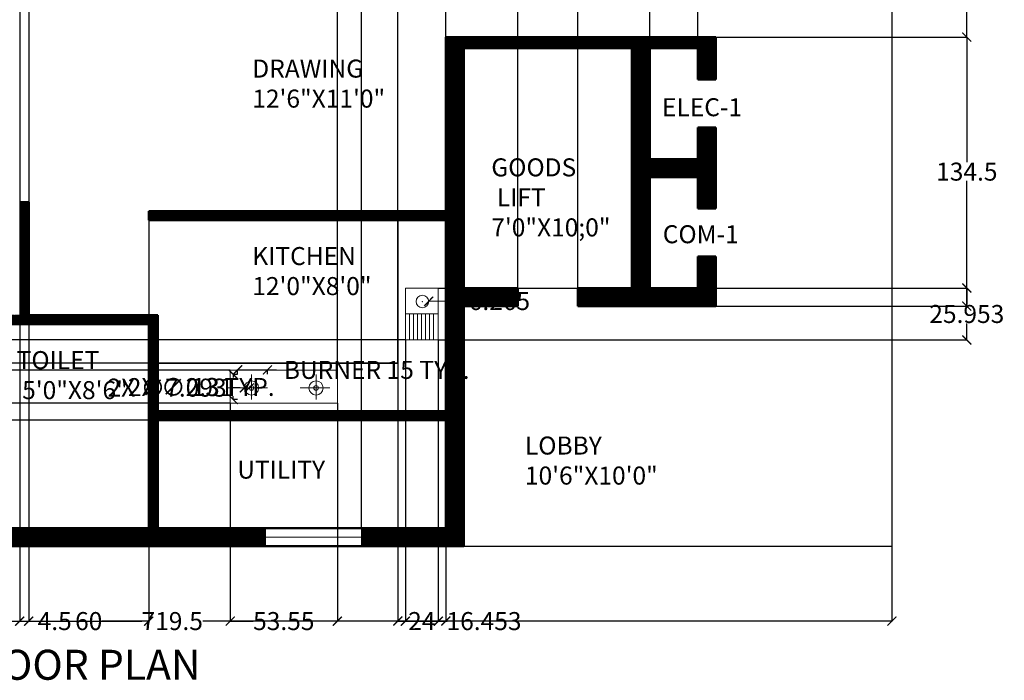
# Model space of a CAD drawing. Units: inches. Extents: x 273 to 1105, y 406 to 1027.
# Tile 2 of 3: x 612 to 1105, y 406 to 736. Entities that reach past the tile are written whole.
import ezdxf

# ---------------------------------------------------------------- set-up
doc = ezdxf.new("R2010")
doc.units = ezdxf.units.IN
doc.header["$MEASUREMENT"] = 0
for name, color, linetype, lineweight in [('A-ANNO-DIMS', 2, 'Continuous', 18), ('A-ANNO-TEXT', 7, 'Continuous', 25), ('A-AREA-IDEN', 7, 'Continuous', 18), ('A-EQPM', 8, 'Continuous', 18), ('A-FIXT-PATT', 8, 'Continuous', 13), ('A-FLOR-CASE', 8, 'Continuous', 25), ('A-FLOR-FIXT', 8, 'Continuous', 18), ('A-FLOR-OTLN', 7, 'Continuous', 25), ('A-GLAZ', 4, 'Continuous', 18), ('A-WALL', 7, 'Continuous', 50), ('A-WALL-PATT', 252, 'Continuous', 13)]:
    doc.layers.add(name, color=color, linetype=linetype, lineweight=lineweight)
doc.styles.get("Standard").update_dxf_attribs({"font": 'arial.ttf'})
doc.dimstyles.get("Standard").update_dxf_attribs({"dimtxt": 9, "dimasz": 4.5, "dimexe": 0.18, "dimexo": 0.0625, "dimgap": 0.09, "dimtad": 0, "dimtih": 1, "dimtoh": 1, "dimdec": 1, "dimzin": 0, "dimdsep": 46, "dimlunit": 4, "dimtxsty": 'Standard', "dimblk": 'ARCHTICK', "dimcen": 0.09, "dimadec": 0, "dimazin": 0, "dimtfac": 1, "dimtdec": 1, "dimtofl": 0, "dimtmove": 0, "dimatfit": 3, "dimfxl": 1, "dimtolj": 1, "dimtzin": 0, "dimarcsym": 0})

# ---------------------------------------------------------------- blocks, each defined once
blk = doc.blocks.new('WIN-48')
for p, q in [((0, 9), (48, 9)), ((0, 0), (0, 9)), ((48, 9), (48, 0)), ((0, 4.5), (48, 4.5)), ((48, 0), (0, 0))]:
    blk.add_line(p, q)
blk = doc.blocks.new('COOKTOP-BURNER')
for p, q in [((6.91, 5.79), (6.91, 12.57)), ((14.89, 5.79), (0, 5.79)), ((0, 5.79), (6.91, 5.79)), ((6.91, 5.79), (6.91, 5.79)), ((6.91, 5.79), (14.89, 5.79)), ((6.91, 5.79), (6.91, 5.79)), ((6.91, 5.79), (6.91, 5.79)), ((6.91, 5.79), (6.91, 5.79)), ((6.91, 5.79), (6.91, 0)), ((6.91, 0), (6.91, 5.79))]:
    blk.add_line(p, q)
for radius in [3.55, 1.16]:
    blk.add_circle((6.91, 5.79), radius)
blk = doc.blocks.new('_ArchTick')
at = {"color": 0, "linetype": 'ByBlock', "const_width": 0.15}
blk.add_lwpolyline([(-0.5, -0.5), (0.5, 0.5)], dxfattribs=at)
blk = doc.blocks.new('*D12')
at = {"layer": 'A-ANNO-DIMS', "color": 0, "lineweight": -2, "transparency": 16777216}
for p, q in [((721.33, 558.55), (721.33, 560.9)), ((721.33, 560.72), (736.23, 560.72)), ((736.23, 558.55), (736.23, 560.9)), ((736.23, 560.72), (740.73, 560.72))]:
    blk.add_line(p, q, dxfattribs=at)
at = {"layer": 'Defpoints', "color": 0, "transparency": 16777216}
for p in [(721.33, 558.49), (736.23, 560.72), (736.23, 558.49)]:
    blk.add_point(p, dxfattribs=at)
at = {"layer": 'A-ANNO-DIMS', "color": 0, "lineweight": -2, "transparency": 16777216, "xscale": 4.5, "yscale": 4.5, "zscale": 4.5, "rotation": 180}
blk.add_blockref('_ArchTick', (721.33, 560.72), dxfattribs=at)
at = {"layer": 'A-ANNO-DIMS', "color": 0, "lineweight": -2, "transparency": 16777216, "xscale": 4.5, "yscale": 4.5, "zscale": 4.5}
blk.add_blockref('_ArchTick', (736.23, 560.72), dxfattribs=at)
at = {"layer": 'A-ANNO-DIMS', "color": 0, "transparency": 16777216, "insert": (790.82, 560.72), "char_height": 9, "attachment_point": 5}
blk.add_mtext('\\A1;BURNER 15 TYP.', dxfattribs=at)
blk = doc.blocks.new('*D13')
at = {"layer": 'A-ANNO-DIMS', "color": 0, "lineweight": -2, "transparency": 16777216}
for p, q in [((721.27, 558.49), (718.92, 558.49)), ((719.1, 558.49), (719.1, 556.89)), ((719.1, 545.92), (719.1, 547.51)), ((721.27, 545.92), (718.92, 545.92))]:
    blk.add_line(p, q, dxfattribs=at)
at = {"layer": 'Defpoints', "color": 0, "transparency": 16777216}
for p in [(719.1, 558.49), (721.33, 558.49), (721.33, 545.92)]:
    blk.add_point(p, dxfattribs=at)
at = {"layer": 'A-ANNO-DIMS', "color": 0, "lineweight": -2, "transparency": 16777216, "xscale": 4.5, "yscale": 4.5, "zscale": 4.5}
for p, rotation in [((719.1, 558.49), 90), ((719.1, 545.92), 270)]:
    blk.add_blockref('_ArchTick', p, dxfattribs=dict(at, rotation=rotation))
at = {"layer": 'A-ANNO-DIMS', "color": 0, "transparency": 16777216, "insert": (719.1, 552.2), "char_height": 9, "attachment_point": 5}
blk.add_mtext('\\A1;13 TYP.', dxfattribs=at)
blk = doc.blocks.new('*D14')
at = {"layer": 'A-ANNO-DIMS', "color": 0, "lineweight": -2, "transparency": 16777216}
for p, q in [((328.87, 472.54), (328.87, 434.97)), ((1048.37, 472.54), (1048.37, 434.97)), ((328.87, 435.15), (673.35, 435.15)), ((1048.37, 435.15), (703.9, 435.15))]:
    blk.add_line(p, q, dxfattribs=at)
at = {"layer": 'Defpoints', "color": 0, "transparency": 16777216}
for p in [(328.87, 472.6), (1048.37, 472.6), (1048.37, 435.15)]:
    blk.add_point(p, dxfattribs=at)
at = {"layer": 'A-ANNO-DIMS', "color": 0, "lineweight": -2, "transparency": 16777216, "xscale": 4.5, "yscale": 4.5, "zscale": 4.5, "rotation": 180}
blk.add_blockref('_ArchTick', (328.87, 435.15), dxfattribs=at)
at = {"layer": 'A-ANNO-DIMS', "color": 0, "lineweight": -2, "transparency": 16777216, "xscale": 4.5, "yscale": 4.5, "zscale": 4.5}
blk.add_blockref('_ArchTick', (1048.37, 435.15), dxfattribs=at)
at = {"layer": 'A-ANNO-DIMS', "color": 0, "transparency": 16777216, "insert": (688.62, 435.15), "char_height": 9, "attachment_point": 5}
blk.add_mtext('\\A1;719.5', dxfattribs=at)
blk = doc.blocks.new('*D22')
at = {"layer": 'A-ANNO-DIMS', "color": 0, "lineweight": -2, "transparency": 16777216}
for p, q in [((960.44, 727.1), (1086, 727.1)), ((1085.82, 727.1), (1085.82, 664.54)), ((1085.82, 592.6), (1085.82, 655.17)), ((960.44, 592.6), (1086, 592.6))]:
    blk.add_line(p, q, dxfattribs=at)
at = {"layer": 'Defpoints', "color": 0, "transparency": 16777216}
for p in [(960.37, 727.1), (1085.82, 727.1), (960.37, 592.6)]:
    blk.add_point(p, dxfattribs=at)
at = {"layer": 'A-ANNO-DIMS', "color": 0, "lineweight": -2, "transparency": 16777216, "xscale": 4.5, "yscale": 4.5, "zscale": 4.5}
for p, rotation in [((1085.82, 727.1), 90), ((1085.82, 592.6), 270)]:
    blk.add_blockref('_ArchTick', p, dxfattribs=dict(at, rotation=rotation))
at = {"layer": 'A-ANNO-DIMS', "color": 0, "transparency": 16777216, "insert": (1085.82, 659.85), "char_height": 9, "attachment_point": 5}
blk.add_mtext('\\A1;134.5', dxfattribs=at)
blk = doc.blocks.new('*D23')
at = {"layer": 'A-ANNO-DIMS', "color": 0, "lineweight": -2, "transparency": 16777216}
for p, q in [((834.44, 763.1), (1086, 763.1)), ((1085.82, 763.1), (1085.82, 749.79)), ((1085.82, 727.1), (1085.82, 740.42)), ((960.44, 727.1), (1086, 727.1))]:
    blk.add_line(p, q, dxfattribs=at)
at = {"layer": 'Defpoints', "color": 0, "transparency": 16777216}
for p in [(834.37, 763.1), (1085.82, 763.1), (960.37, 727.1)]:
    blk.add_point(p, dxfattribs=at)
at = {"layer": 'A-ANNO-DIMS', "color": 0, "lineweight": -2, "transparency": 16777216, "xscale": 4.5, "yscale": 4.5, "zscale": 4.5}
for p, rotation in [((1085.82, 763.1), 90), ((1085.82, 727.1), 270)]:
    blk.add_blockref('_ArchTick', p, dxfattribs=dict(at, rotation=rotation))
at = {"layer": 'A-ANNO-DIMS', "color": 0, "transparency": 16777216, "insert": (1085.82, 745.1), "char_height": 9, "attachment_point": 5}
blk.add_mtext('\\A1;36', dxfattribs=at)
blk = doc.blocks.new('*D25')
at = {"layer": 'A-ANNO-DIMS', "color": 0, "lineweight": -2, "transparency": 16777216}
for p, q in [((927.37, 721.67), (927.37, 1021.23)), ((927.37, 1021.05), (932.78, 1021.05)), ((951.37, 1021.05), (945.97, 1021.05)), ((951.37, 721.67), (951.37, 1021.23))]:
    blk.add_line(p, q, dxfattribs=at)
at = {"layer": 'Defpoints', "color": 0, "transparency": 16777216}
for p in [(951.37, 1021.05), (927.37, 721.6), (951.37, 721.6)]:
    blk.add_point(p, dxfattribs=at)
at = {"layer": 'A-ANNO-DIMS', "color": 0, "lineweight": -2, "transparency": 16777216, "xscale": 4.5, "yscale": 4.5, "zscale": 4.5, "rotation": 180}
blk.add_blockref('_ArchTick', (927.37, 1021.05), dxfattribs=at)
at = {"layer": 'A-ANNO-DIMS', "color": 0, "lineweight": -2, "transparency": 16777216, "xscale": 4.5, "yscale": 4.5, "zscale": 4.5}
blk.add_blockref('_ArchTick', (951.37, 1021.05), dxfattribs=at)
at = {"layer": 'A-ANNO-DIMS', "color": 0, "transparency": 16777216, "insert": (939.37, 1021.05), "char_height": 9, "attachment_point": 5}
blk.add_mtext('\\A1;24', dxfattribs=at)
blk = doc.blocks.new('*D26')
at = {"layer": 'A-ANNO-DIMS', "color": 0, "lineweight": -2, "transparency": 16777216}
for p, q in [((861.37, 592.67), (861.37, 1021.23)), ((861.37, 1021.05), (869.86, 1021.05)), ((891.37, 1021.05), (882.89, 1021.05)), ((891.37, 592.67), (891.37, 1021.23))]:
    blk.add_line(p, q, dxfattribs=at)
at = {"layer": 'Defpoints', "color": 0, "transparency": 16777216}
for p in [(891.37, 1021.05), (861.37, 592.6), (891.37, 592.6)]:
    blk.add_point(p, dxfattribs=at)
at = {"layer": 'A-ANNO-DIMS', "color": 0, "lineweight": -2, "transparency": 16777216, "xscale": 4.5, "yscale": 4.5, "zscale": 4.5, "rotation": 180}
blk.add_blockref('_ArchTick', (861.37, 1021.05), dxfattribs=at)
at = {"layer": 'A-ANNO-DIMS', "color": 0, "lineweight": -2, "transparency": 16777216, "xscale": 4.5, "yscale": 4.5, "zscale": 4.5}
blk.add_blockref('_ArchTick', (891.37, 1021.05), dxfattribs=at)
at = {"layer": 'A-ANNO-DIMS', "color": 0, "transparency": 16777216, "insert": (876.37, 1021.05), "char_height": 9, "attachment_point": 5}
blk.add_mtext('\\A1;30', dxfattribs=at)
blk = doc.blocks.new('*D27')
at = {"layer": 'A-ANNO-DIMS', "color": 0, "lineweight": -2, "transparency": 16777216}
for p, q in [((825.31, 535.6), (291.24, 535.6)), ((291.42, 535.6), (291.42, 513.27)), ((291.42, 481.6), (291.42, 503.94)), ((825.31, 481.6), (291.24, 481.6))]:
    blk.add_line(p, q, dxfattribs=at)
at = {"layer": 'Defpoints', "color": 0, "transparency": 16777216}
for p in [(291.42, 535.6), (825.37, 535.6), (825.37, 481.6)]:
    blk.add_point(p, dxfattribs=at)
at = {"layer": 'A-ANNO-DIMS', "color": 0, "lineweight": -2, "transparency": 16777216, "xscale": 4.5, "yscale": 4.5, "zscale": 4.5}
for p, rotation in [((291.42, 535.6), 90), ((291.42, 481.6), 270)]:
    blk.add_blockref('_ArchTick', p, dxfattribs=dict(at, rotation=rotation))
at = {"layer": 'A-ANNO-DIMS', "color": 0, "transparency": 16777216, "insert": (291.42, 508.6), "char_height": 9, "attachment_point": 5}
blk.add_mtext('\\A1;54', dxfattribs=at)
blk = doc.blocks.new('*D28')
at = {"layer": 'A-ANNO-DIMS', "color": 0, "lineweight": -2, "transparency": 16777216}
for p, q in [((783.25, 481.67), (783.25, 1021.23)), ((783.25, 1021.05), (788.85, 1021.05)), ((825.37, 1021.05), (819.77, 1021.05)), ((825.37, 481.67), (825.37, 1021.23))]:
    blk.add_line(p, q, dxfattribs=at)
at = {"layer": 'Defpoints', "color": 0, "transparency": 16777216}
for p in [(825.37, 1021.05), (783.25, 481.6), (825.37, 481.6)]:
    blk.add_point(p, dxfattribs=at)
at = {"layer": 'A-ANNO-DIMS', "color": 0, "lineweight": -2, "transparency": 16777216, "xscale": 4.5, "yscale": 4.5, "zscale": 4.5, "rotation": 180}
blk.add_blockref('_ArchTick', (783.25, 1021.05), dxfattribs=at)
at = {"layer": 'A-ANNO-DIMS', "color": 0, "lineweight": -2, "transparency": 16777216, "xscale": 4.5, "yscale": 4.5, "zscale": 4.5}
blk.add_blockref('_ArchTick', (825.37, 1021.05), dxfattribs=at)
at = {"layer": 'A-ANNO-DIMS', "color": 0, "transparency": 16777216, "insert": (804.31, 1021.05), "char_height": 9, "attachment_point": 5}
blk.add_mtext('\\A1;42.13', dxfattribs=at)
blk = doc.blocks.new('*D29')
at = {"layer": 'A-ANNO-DIMS', "color": 0, "lineweight": -2, "transparency": 16777216}
for p, q in [((801.37, 635.54), (801.37, 434.97)), ((825.37, 635.54), (825.37, 434.97)), ((801.37, 435.15), (806.78, 435.15)), ((825.37, 435.15), (819.97, 435.15))]:
    blk.add_line(p, q, dxfattribs=at)
at = {"layer": 'Defpoints', "color": 0, "transparency": 16777216}
for p in [(801.37, 635.6), (825.37, 635.6), (825.37, 435.15)]:
    blk.add_point(p, dxfattribs=at)
at = {"layer": 'A-ANNO-DIMS', "color": 0, "lineweight": -2, "transparency": 16777216, "xscale": 4.5, "yscale": 4.5, "zscale": 4.5, "rotation": 180}
blk.add_blockref('_ArchTick', (801.37, 435.15), dxfattribs=at)
at = {"layer": 'A-ANNO-DIMS', "color": 0, "lineweight": -2, "transparency": 16777216, "xscale": 4.5, "yscale": 4.5, "zscale": 4.5}
blk.add_blockref('_ArchTick', (825.37, 435.15), dxfattribs=at)
at = {"layer": 'A-ANNO-DIMS', "color": 0, "transparency": 16777216, "insert": (813.37, 435.15), "char_height": 9, "attachment_point": 5}
blk.add_mtext('\\A1;24', dxfattribs=at)
blk = doc.blocks.new('*D31')
at = {"layer": 'A-ANNO-DIMS', "color": 0, "lineweight": -2, "transparency": 16777216}
for p, q in [((612.37, 820.54), (612.37, 434.97)), ((616.87, 820.54), (616.87, 434.97)), ((612.37, 435.15), (616.87, 435.15)), ((616.87, 435.15), (621.37, 435.15))]:
    blk.add_line(p, q, dxfattribs=at)
at = {"layer": 'Defpoints', "color": 0, "transparency": 16777216}
for p in [(612.37, 820.6), (616.87, 820.6), (616.87, 435.15)]:
    blk.add_point(p, dxfattribs=at)
at = {"layer": 'A-ANNO-DIMS', "color": 0, "lineweight": -2, "transparency": 16777216, "xscale": 4.5, "yscale": 4.5, "zscale": 4.5, "rotation": 180}
blk.add_blockref('_ArchTick', (612.37, 435.15), dxfattribs=at)
at = {"layer": 'A-ANNO-DIMS', "color": 0, "lineweight": -2, "transparency": 16777216, "xscale": 4.5, "yscale": 4.5, "zscale": 4.5}
blk.add_blockref('_ArchTick', (616.87, 435.15), dxfattribs=at)
at = {"layer": 'A-ANNO-DIMS', "color": 0, "transparency": 16777216, "insert": (629.87, 435.15), "char_height": 9, "attachment_point": 5}
blk.add_mtext('\\A1;4.5', dxfattribs=at)
blk = doc.blocks.new('*D33')
at = {"layer": 'A-ANNO-DIMS', "color": 0, "lineweight": -2, "transparency": 16777216}
for p, q in [((616.87, 644.54), (616.87, 434.97)), ((676.87, 640.04), (676.87, 434.97)), ((616.87, 435.15), (640.33, 435.15)), ((676.87, 435.15), (653.42, 435.15))]:
    blk.add_line(p, q, dxfattribs=at)
at = {"layer": 'Defpoints', "color": 0, "transparency": 16777216}
for p in [(616.87, 644.6), (676.87, 640.1), (676.87, 435.15)]:
    blk.add_point(p, dxfattribs=at)
at = {"layer": 'A-ANNO-DIMS', "color": 0, "lineweight": -2, "transparency": 16777216, "xscale": 4.5, "yscale": 4.5, "zscale": 4.5, "rotation": 180}
blk.add_blockref('_ArchTick', (616.87, 435.15), dxfattribs=at)
at = {"layer": 'A-ANNO-DIMS', "color": 0, "lineweight": -2, "transparency": 16777216, "xscale": 4.5, "yscale": 4.5, "zscale": 4.5}
blk.add_blockref('_ArchTick', (676.87, 435.15), dxfattribs=at)
at = {"layer": 'A-ANNO-DIMS', "color": 0, "transparency": 16777216, "insert": (646.87, 435.15), "char_height": 9, "attachment_point": 5}
blk.add_mtext('\\A1;60', dxfattribs=at)
blk = doc.blocks.new('*D34')
at = {"layer": 'A-ANNO-DIMS', "color": 0, "lineweight": -2, "transparency": 16777216}
for p, q in [((717.61, 544.02), (717.61, 434.97)), ((771.16, 544.02), (771.16, 434.97)), ((717.61, 435.15), (729.08, 435.15)), ((771.16, 435.15), (759.69, 435.15))]:
    blk.add_line(p, q, dxfattribs=at)
at = {"layer": 'Defpoints', "color": 0, "transparency": 16777216}
for p in [(717.61, 544.09), (771.16, 544.09), (771.16, 435.15)]:
    blk.add_point(p, dxfattribs=at)
at = {"layer": 'A-ANNO-DIMS', "color": 0, "lineweight": -2, "transparency": 16777216, "xscale": 4.5, "yscale": 4.5, "zscale": 4.5, "rotation": 180}
blk.add_blockref('_ArchTick', (717.61, 435.15), dxfattribs=at)
at = {"layer": 'A-ANNO-DIMS', "color": 0, "lineweight": -2, "transparency": 16777216, "xscale": 4.5, "yscale": 4.5, "zscale": 4.5}
blk.add_blockref('_ArchTick', (771.16, 435.15), dxfattribs=at)
at = {"layer": 'A-ANNO-DIMS', "color": 0, "transparency": 16777216, "insert": (744.39, 435.15), "char_height": 9, "attachment_point": 5}
blk.add_mtext('\\A1;53.55', dxfattribs=at)
blk = doc.blocks.new('*D35')
at = {"layer": 'A-ANNO-DIMS', "color": 0, "lineweight": -2, "transparency": 16777216}
for p, q in [((717.55, 560.57), (291.24, 560.57)), ((291.42, 560.57), (291.42, 557.01)), ((291.42, 544.09), (291.42, 547.64)), ((717.55, 544.09), (291.24, 544.09))]:
    blk.add_line(p, q, dxfattribs=at)
at = {"layer": 'Defpoints', "color": 0, "transparency": 16777216}
for p in [(717.61, 560.57), (291.42, 544.09), (717.61, 544.09)]:
    blk.add_point(p, dxfattribs=at)
at = {"layer": 'A-ANNO-DIMS', "color": 0, "lineweight": -2, "transparency": 16777216, "xscale": 4.5, "yscale": 4.5, "zscale": 4.5}
for p, rotation in [((291.42, 560.57), 90), ((291.42, 544.09), 270)]:
    blk.add_blockref('_ArchTick', p, dxfattribs=dict(at, rotation=rotation))
at = {"layer": 'A-ANNO-DIMS', "color": 0, "transparency": 16777216, "insert": (291.42, 552.33), "char_height": 9, "attachment_point": 5}
blk.add_mtext('\\A1;16.482', dxfattribs=at)
blk = doc.blocks.new('*D36')
at = {"layer": 'A-ANNO-DIMS', "color": 0, "lineweight": -2, "transparency": 16777216}
for p, q in [((821.69, 601.66), (1086, 601.66)), ((1085.82, 601.66), (1085.82, 593.37)), ((1085.82, 575.7), (1085.82, 583.99)), ((821.69, 575.7), (1086, 575.7))]:
    blk.add_line(p, q, dxfattribs=at)
at = {"layer": 'Defpoints', "color": 0, "transparency": 16777216}
for p in [(821.63, 601.66), (1085.82, 601.66), (821.63, 575.7)]:
    blk.add_point(p, dxfattribs=at)
at = {"layer": 'A-ANNO-DIMS', "color": 0, "lineweight": -2, "transparency": 16777216, "xscale": 4.5, "yscale": 4.5, "zscale": 4.5}
for p, rotation in [((1085.82, 601.66), 90), ((1085.82, 575.7), 270)]:
    blk.add_blockref('_ArchTick', p, dxfattribs=dict(at, rotation=rotation))
at = {"layer": 'A-ANNO-DIMS', "color": 0, "transparency": 16777216, "insert": (1085.82, 588.68), "char_height": 9, "attachment_point": 5}
blk.add_mtext('\\A1;25.953', dxfattribs=at)
blk = doc.blocks.new('*D37')
at = {"layer": 'A-ANNO-DIMS', "color": 0, "lineweight": -2, "transparency": 16777216}
for p, q in [((805.18, 575.64), (805.18, 434.97)), ((821.63, 575.64), (821.63, 434.97)), ((805.18, 435.15), (821.63, 435.15)), ((821.63, 435.15), (826.13, 435.15))]:
    blk.add_line(p, q, dxfattribs=at)
at = {"layer": 'Defpoints', "color": 0, "transparency": 16777216}
for p in [(805.18, 575.7), (821.63, 575.7), (821.63, 435.15)]:
    blk.add_point(p, dxfattribs=at)
at = {"layer": 'A-ANNO-DIMS', "color": 0, "lineweight": -2, "transparency": 16777216, "xscale": 4.5, "yscale": 4.5, "zscale": 4.5, "rotation": 180}
blk.add_blockref('_ArchTick', (805.18, 435.15), dxfattribs=at)
at = {"layer": 'A-ANNO-DIMS', "color": 0, "lineweight": -2, "transparency": 16777216, "xscale": 4.5, "yscale": 4.5, "zscale": 4.5}
blk.add_blockref('_ArchTick', (821.63, 435.15), dxfattribs=at)
at = {"layer": 'A-ANNO-DIMS', "color": 0, "transparency": 16777216, "insert": (844.48, 435.15), "char_height": 9, "attachment_point": 5}
blk.add_mtext('\\A1;16.453', dxfattribs=at)
blk = doc.blocks.new('*D38')
at = {"layer": 'A-ANNO-DIMS', "color": 0, "lineweight": -2, "transparency": 16777216}
for p, q in [((771.16, 560.63), (771.16, 1021.23)), ((771.16, 1021.05), (801.37, 1021.05)), ((801.37, 564.17), (801.37, 1021.23)), ((801.37, 1021.05), (805.87, 1021.05))]:
    blk.add_line(p, q, dxfattribs=at)
at = {"layer": 'Defpoints', "color": 0, "transparency": 16777216}
for p in [(801.37, 1021.05), (801.37, 564.1), (771.16, 560.57)]:
    blk.add_point(p, dxfattribs=at)
at = {"layer": 'A-ANNO-DIMS', "color": 0, "lineweight": -2, "transparency": 16777216, "xscale": 4.5, "yscale": 4.5, "zscale": 4.5, "rotation": 180}
blk.add_blockref('_ArchTick', (771.16, 1021.05), dxfattribs=at)
at = {"layer": 'A-ANNO-DIMS', "color": 0, "lineweight": -2, "transparency": 16777216, "xscale": 4.5, "yscale": 4.5, "zscale": 4.5}
blk.add_blockref('_ArchTick', (801.37, 1021.05), dxfattribs=at)
at = {"layer": 'A-ANNO-DIMS', "color": 0, "transparency": 16777216, "insert": (824.68, 1021.05), "char_height": 9, "attachment_point": 5}
blk.add_mtext('\\A1;30.215', dxfattribs=at)
blk = doc.blocks.new('*D39')
at = {"layer": 'A-ANNO-DIMS', "color": 0, "lineweight": -2, "transparency": 16777216}
for p, q in [((805.12, 575.7), (291.24, 575.7)), ((291.42, 575.7), (291.42, 574.59)), ((801.31, 564.1), (291.24, 564.1)), ((291.42, 564.1), (291.42, 565.22))]:
    blk.add_line(p, q, dxfattribs=at)
at = {"layer": 'Defpoints', "color": 0, "transparency": 16777216}
for p in [(291.42, 575.7), (805.18, 575.7), (801.37, 564.1)]:
    blk.add_point(p, dxfattribs=at)
at = {"layer": 'A-ANNO-DIMS', "color": 0, "lineweight": -2, "transparency": 16777216, "xscale": 4.5, "yscale": 4.5, "zscale": 4.5}
for p, rotation in [((291.42, 575.7), 90), ((291.42, 564.1), 270)]:
    blk.add_blockref('_ArchTick', p, dxfattribs=dict(at, rotation=rotation))
at = {"layer": 'A-ANNO-DIMS', "color": 0, "transparency": 16777216, "insert": (291.42, 569.9), "char_height": 9, "attachment_point": 5}
blk.add_mtext('\\A1;11.6', dxfattribs=at)
blk = doc.blocks.new('*D41')
at = {"layer": 'A-ANNO-DIMS', "color": 0, "lineweight": -2, "transparency": 16777216}
for p, q in [((813.59, 594.95), (813.77, 594.95)), ((813.68, 594.86), (813.68, 595.04)), ((825.81, 595.15), (816.82, 595))]:
    blk.add_line(p, q, dxfattribs=at)
at = {"layer": 'Defpoints', "color": 0, "transparency": 16777216}
for p in [(810.55, 594.89), (816.82, 595)]:
    blk.add_point(p, dxfattribs=at)
at = {"layer": 'A-ANNO-DIMS', "color": 0, "lineweight": -2, "transparency": 16777216, "xscale": 4.5, "yscale": 4.5, "zscale": 4.5, "rotation": 180.9882264643174}
blk.add_blockref('_ArchTick', (816.82, 595), dxfattribs=at)
at = {"layer": 'A-ANNO-DIMS', "color": 0, "transparency": 16777216, "insert": (846.02, 595.15), "char_height": 9, "attachment_point": 5}
blk.add_mtext('\\A1;∅6.265', dxfattribs=at)
blk = doc.blocks.new('*D42')
at = {"layer": 'A-ANNO-DIMS', "color": 0, "lineweight": -2, "transparency": 16777216}
for p, q in [((715.7, 551.86), (724.7, 551.75)), ((728.16, 551.71), (728.34, 551.71)), ((728.25, 551.62), (728.25, 551.8))]:
    blk.add_line(p, q, dxfattribs=at)
at = {"layer": 'Defpoints', "color": 0, "transparency": 16777216}
for p in [(724.7, 551.75), (731.8, 551.66)]:
    blk.add_point(p, dxfattribs=at)
at = {"layer": 'A-ANNO-DIMS', "color": 0, "lineweight": -2, "transparency": 16777216, "xscale": 4.5, "yscale": 4.5, "zscale": 4.5, "rotation": 359.2861452367267}
blk.add_blockref('_ArchTick', (724.7, 551.75), dxfattribs=at)
at = {"layer": 'A-ANNO-DIMS', "color": 0, "transparency": 16777216, "insert": (686.03, 551.86), "char_height": 9, "attachment_point": 5}
blk.add_mtext('\\A1;2X ∅7.093', dxfattribs=at)
blk = doc.blocks.new('*D43')
at = {"layer": 'A-ANNO-DIMS', "color": 0, "lineweight": -2, "transparency": 16777216}
for p, q in [((718.1, 552.11), (727.1, 551.75)), ((728.16, 551.71), (728.34, 551.71)), ((728.25, 551.62), (728.25, 551.8))]:
    blk.add_line(p, q, dxfattribs=at)
at = {"layer": 'Defpoints', "color": 0, "transparency": 16777216}
for p in [(727.1, 551.75), (729.4, 551.66)]:
    blk.add_point(p, dxfattribs=at)
at = {"layer": 'A-ANNO-DIMS', "color": 0, "lineweight": -2, "transparency": 16777216, "xscale": 4.5, "yscale": 4.5, "zscale": 4.5, "rotation": 357.7230243181089}
blk.add_blockref('_ArchTick', (727.1, 551.75), dxfattribs=at)
at = {"layer": 'A-ANNO-DIMS', "color": 0, "transparency": 16777216, "insert": (692.79, 552.11), "char_height": 9, "attachment_point": 5}
blk.add_mtext('\\A1;2X ∅2.31', dxfattribs=at)

msp = doc.modelspace()

# ---------------------------------------------------------------- hatches: boundary and pattern name
at = {"layer": 'A-FIXT-PATT'}
h = msp.add_hatch(dxfattribs=at)
h.set_pattern_fill('ANSI31', color=256, scale=15.9837, angle=45, style=0)
h.paths.add_polyline_path([(806.1776, 575.7043), (820.1776, 575.7043), (820.1776, 588.6809), (806.1776, 588.6809)])
at = {"layer": 'A-WALL-PATT'}
h = msp.add_hatch(dxfattribs=at)
h.set_pattern_fill('ANSI31', color=256)
h.paths.add_polyline_path([(735.2471, 481.6046), (681.3741, 481.6046), (681.3741, 535.6046), (825.3741, 535.6046), (825.3741, 481.6046), (783.2471, 481.6046), (783.2471, 472.6046), (834.3741, 472.6046), (834.3741, 592.6046), (861.3741, 592.6046), (861.3741, 601.6046), (834.3741, 601.6046), (834.3741, 721.6046), (918.3741, 721.6046), (918.3741, 601.6046), (891.3741, 601.6046), (891.3741, 592.6046), (960.3741, 592.6046), (960.3741, 617.3546), (951.3741, 617.3546), (951.3741, 601.6046), (927.3741, 601.6046), (927.3741, 657.1046), (951.3741, 657.1046), (951.3741, 641.3546), (960.3741, 641.3546), (960.3741, 681.8546), (951.3741, 681.8546), (951.3741, 666.1046), (927.3741, 666.1046), (927.3741, 721.6046), (951.3741, 721.6046), (951.3741, 705.8546), (960.3741, 705.8546), (960.3741, 727.1046), (834.3741, 727.1046), (825.3741, 727.1046), (825.3741, 640.1046), (681.3741, 640.1046), (676.8741, 640.1046), (676.8741, 635.6046), (681.3741, 635.6046), (825.3741, 635.6046), (825.3741, 540.1046), (681.3741, 540.1046), (681.3741, 588.1046), (676.8741, 588.1046), (616.8741, 588.1046), (616.8741, 644.6046), (612.3741, 644.6046), (612.3741, 640.1046), (612.3741, 588.1046), (552.3741, 588.1046), (552.3741, 640.1046), (552.3741, 644.6046), (547.8741, 644.6046), (547.8741, 640.1046), (547.8741, 635.6046), (547.8741, 547.6046), (552.3741, 547.6046), (552.3741, 583.6046), (602.3741, 583.6046), (602.3741, 547.6046), (606.8741, 547.6046), (606.8741, 583.6046), (676.8741, 583.6046), (676.8741, 481.6046), (552.3741, 481.6046), (552.3741, 517.6046), (547.8741, 517.6046), (547.8741, 481.6046), (493.8741, 481.6046), (493.8741, 472.6046), (547.8741, 472.6046), (735.2471, 472.6046)])
h.paths.add_polyline_path([(445.8741, 481.6046), (391.8741, 481.6046), (391.8741, 576.6354), (382.8741, 576.6354), (382.8741, 472.6046), (391.8741, 472.6046), (445.8741, 472.6046)])
h.paths.add_polyline_path([(729.3741, 929.6046), (658.8741, 929.6046), (658.8741, 920.6046), (676.8741, 920.6046), (676.8741, 916.1046), (681.3741, 916.1046), (681.3741, 920.6046), (729.3741, 920.6046)])
h.paths.add_polyline_path([(834.3741, 929.6046), (777.3741, 929.6046), (777.3741, 920.6046), (825.3741, 920.6046), (825.3741, 776.6046), (681.3741, 776.6046), (676.8741, 776.6046), (676.8741, 772.1046), (681.3741, 772.1046), (825.3741, 772.1046), (825.3741, 763.1046), (834.3741, 763.1046)])
h.paths.add_polyline_path([(1048.3741, 850.6046), (834.3741, 850.6046), (834.3741, 841.6046), (1048.3741, 841.6046)])
h.paths.add_polyline_path([(337.8741, 772.1046), (391.8741, 772.1046), (415.8741, 772.1046), (420.3741, 772.1046), (424.8741, 772.1046), (547.8741, 772.1046), (547.8741, 774.3546), (424.8741, 774.3546), (424.8741, 776.6046), (391.8741, 776.6046), (391.8741, 920.6046), (445.8741, 920.6046), (445.8741, 929.6046), (382.8741, 929.6046), (382.8741, 776.6046), (328.8741, 776.6046), (328.8741, 772.1046), (328.8741, 635.6046), (382.8741, 635.6046), (391.8741, 635.6046), (424.8741, 635.6046), (511.8741, 635.6046), (511.8741, 640.1046), (415.8741, 640.1046), (391.8741, 640.1046), (337.8741, 640.1046)])
h.paths.add_polyline_path([(570.3741, 929.6046), (493.8741, 929.6046), (493.8741, 920.6046), (547.8741, 920.6046), (547.8741, 916.1046), (552.3741, 916.1046), (552.3741, 920.6046), (570.3741, 920.6046)])
h.paths.add_polyline_path([(634.8741, 929.6046), (594.3741, 929.6046), (594.3741, 920.6046), (612.3741, 920.6046), (612.3741, 820.6046), (552.3741, 820.6046), (552.3741, 886.1046), (547.8741, 886.1046), (547.8741, 816.1046), (552.3741, 816.1046), (612.3741, 816.1046), (616.8741, 816.1046), (676.8741, 816.1046), (681.3741, 816.1046), (681.3741, 886.1046), (676.8741, 886.1046), (676.8741, 820.6046), (616.8741, 820.6046), (616.8741, 920.6046), (634.8741, 920.6046)])

# ---------------------------------------------------------------- linework, layer by layer
at = {"layer": 'A-EQPM'}
for p, q in [((717.6111, 560.5674), (771.1596, 560.5674)), ((717.6111, 544.0857), (717.6111, 560.5674)), ((771.1596, 560.5674), (771.1596, 544.0857)), ((771.1596, 544.0857), (717.6111, 544.0857))]:
    msp.add_line(p, q, dxfattribs=at)
at = {"layer": 'A-FLOR-CASE'}
for p in [(801.3741, 635.6046), (681.3741, 564.1046)]:
    msp.add_line(p, (801.3741, 564.1046), dxfattribs=at)
at = {"layer": 'A-FLOR-FIXT'}
for p, q in [((805.1776, 601.6574), (821.6303, 601.6574)), ((805.1776, 575.7043), (805.1776, 601.6574)), ((821.6303, 601.6574), (821.6303, 575.7043)), ((805.1776, 588.6809), (821.6303, 588.6809)), ((821.6303, 575.7043), (805.1776, 575.7043))]:
    msp.add_line(p, q, dxfattribs=at)
msp.add_circle((813.6838, 594.9454), 3.1323, dxfattribs=at)
at = {"layer": 'A-FLOR-OTLN'}
for p, q in [((1048.3741, 763.1046), (1048.3741, 724.6658)), ((1048.3741, 727.1046), (1048.3741, 472.6046)), ((834.3741, 472.6046), (1048.3741, 472.6046))]:
    msp.add_line(p, q, dxfattribs=at)
at = {"layer": 'A-WALL'}
for p, q in [((825.3741, 727.1046), (834.3741, 727.1046)), ((825.3741, 727.1046), (825.3741, 640.1046)), ((960.3741, 727.1046), (834.3741, 727.1046)), ((960.3741, 727.1046), (960.3741, 705.8546)), ((834.3741, 721.6046), (834.3741, 601.6046)), ((834.3741, 721.6046), (918.3741, 721.6046)), ((918.3741, 721.6046), (918.3741, 601.6046)), ((927.3741, 721.6046), (927.3741, 666.1046)), ((927.3741, 721.6046), (951.3741, 721.6046)), ((951.3741, 721.6046), (951.3741, 705.8546)), ((951.3741, 705.8546), (960.3741, 705.8546)), ((951.3741, 681.8546), (960.3741, 681.8546)), ((951.3741, 681.8546), (951.3741, 666.1046)), ((960.3741, 681.8546), (960.3741, 641.3546)), ((927.3741, 666.1046), (951.3741, 666.1046)), ((927.3741, 657.1046), (951.3741, 657.1046)), ((927.3741, 657.1046), (927.3741, 601.6046)), ((951.3741, 657.1046), (951.3741, 641.3546)), ((612.3741, 644.6046), (616.8741, 644.6046)), ((616.8741, 644.6046), (616.8741, 588.1046)), ((681.3741, 640.1046), (676.8741, 640.1046)), ((676.8741, 640.1046), (676.8741, 635.6046)), ((681.3741, 640.1046), (825.3741, 640.1046)), ((951.3741, 641.3546), (960.3741, 641.3546)), ((681.3741, 635.6046), (676.8741, 635.6046)), ((681.3741, 635.6046), (825.3741, 635.6046)), ((825.3741, 635.6046), (825.3741, 540.1046)), ((951.3741, 617.3546), (960.3741, 617.3546)), ((951.3741, 617.3546), (951.3741, 601.6046)), ((960.3741, 617.3546), (960.3741, 592.6046)), ((834.3741, 601.6046), (861.3741, 601.6046)), ((861.3741, 601.6046), (861.3741, 592.6046)), ((891.3741, 601.6046), (891.3741, 592.6046)), ((891.3741, 601.6046), (918.3741, 601.6046)), ((927.3741, 601.6046), (951.3741, 601.6046)), ((834.3741, 592.6046), (861.3741, 592.6046)), ((834.3741, 592.6046), (834.3741, 472.6046)), ((891.3741, 592.6046), (960.3741, 592.6046)), ((616.8741, 588.1046), (676.8741, 588.1046)), ((676.8741, 588.1046), (681.3741, 588.1046)), ((681.3741, 588.1046), (681.3741, 540.1046)), ((606.8741, 583.6046), (676.8741, 583.6046)), ((676.8741, 583.6046), (676.8741, 481.6046)), ((681.3741, 540.1046), (825.3741, 540.1046)), ((681.3741, 535.6046), (825.3741, 535.6046)), ((681.3741, 535.6046), (681.3741, 481.6046)), ((825.3741, 535.6046), (825.3741, 481.6046)), ((552.3741, 481.6046), (676.8741, 481.6046)), ((681.3741, 481.6046), (825.3741, 481.6046)), ((547.8741, 472.6046), (834.3741, 472.6046))]:
    msp.add_line(p, q, dxfattribs=at)

# ---------------------------------------------------------------- block references
at = {"layer": 'A-EQPM'}
msp.add_blockref('COOKTOP-BURNER', (721.335, 545.915), dxfattribs=at)
at = {"layer": 'A-EQPM', "extrusion": (0, 0, -1), "zscale": -1}
msp.add_blockref('COOKTOP-BURNER', (-767.4356, 545.915), dxfattribs=at)
at = {"layer": 'A-GLAZ'}
msp.add_blockref('WIN-48', (735.2471, 472.605), dxfattribs=at)

# ---------------------------------------------------------------- texts
at = {"layer": 'A-ANNO-TEXT', "insert": (490.6396, 420.8046), "char_height": 15, "attachment_point": 1}
msp.add_mtext_dynamic_manual_height_columns('GROUND FLOOR PLAN', width=435.167248, gutter_width=1, heights=[0], dxfattribs=at)
at = {"layer": 'A-AREA-IDEN', "char_height": 9, "attachment_point": 1}
for s, insert in [('DRAWING\\P12\'6"X11\'0"', (728.6564, 715.8554)), ('ELEC-1', (933.4471, 696.547)), ('GOODS\\P LIFT\\P7\'0"X10;0"', (848.1231, 666.4792)), (' COM-1', (931.085, 633.0501)), ('KITCHEN\\P12\'0"X8\'0"', (728.6564, 622.1363)), ('TOILET\\P 5\'0"X8\'6"', (610.8677, 570.119)), ('LOBBY\\P10\'6"X10\'0"', (864.9395, 527.4045)), ('UTILITY', (721.1085, 515.3431))]:
    msp.add_mtext_dynamic_manual_height_columns(s, width=435.167248, gutter_width=1, heights=[0], dxfattribs=dict(at, insert=insert))

# ---------------------------------------------------------------- dimensions: what is measured, and where the dimension line sits
at = {"layer": 'A-ANNO-DIMS'}
for base, p1, p2, override, picture, middle in [((801.37409, 1021.05461), (771.15955, 560.56745), (801.37409, 564.1046), {"dimdec": 3, "dimlfac": 1, "dimrnd": 0, "dimzin": 0, "dimdsep": 46, "dimlunit": 2}, '*D38', (824.67623, 1021.05461)), ((825.3741, 1021.0546), (783.2471, 481.6046), (825.3741, 481.6046), {"dimdec": 2, "dimlfac": 1, "dimrnd": 0, "dimzin": 0, "dimdsep": 46, "dimlunit": 2}, '*D28', (804.3106, 1021.0546)), ((891.3741, 1021.0546), (861.3741, 592.6046), (891.3741, 592.6046), {"dimdec": 0, "dimlfac": 1, "dimrnd": 0, "dimzin": 0, "dimdsep": 46, "dimlunit": 2}, '*D26', (876.3741, 1021.0546)), ((951.3741, 1021.0546), (927.3741, 721.6046), (951.3741, 721.6046), {"dimdec": 0, "dimlfac": 1, "dimrnd": 0, "dimzin": 0, "dimdsep": 46, "dimlunit": 2}, '*D25', (939.3741, 1021.0546)), ((616.8741, 435.1546), (612.3741, 820.6046), (616.8741, 820.6046), {"dimdec": 1, "dimlfac": 1, "dimrnd": 0, "dimzin": 0, "dimdsep": 46, "dimlunit": 2}, '*D31', (629.8717, 435.1546)), ((676.8741, 435.1546), (616.8741, 644.6046), (676.8741, 640.1046), {"dimdec": 0, "dimlfac": 1, "dimrnd": 0, "dimzin": 0, "dimdsep": 46, "dimlunit": 2}, '*D33', (646.8741, 435.1546)), ((825.3741, 435.1546), (801.3741, 635.6046), (825.3741, 635.6046), {"dimdec": 0, "dimlfac": 1, "dimrnd": 0, "dimzin": 0, "dimdsep": 46, "dimlunit": 2}, '*D29', (813.3741, 435.1546)), ((821.6303, 435.1546), (805.1776, 575.7043), (821.6303, 575.7043), {"dimdec": 3, "dimlfac": 1, "dimrnd": 0, "dimzin": 0, "dimdsep": 46, "dimlunit": 2}, '*D37', (844.4781, 435.1546)), ((771.1596, 435.1546), (717.6111, 544.0857), (771.1596, 544.0857), {"dimdec": 2, "dimlfac": 1, "dimrnd": 0, "dimzin": 0, "dimdsep": 46, "dimlunit": 2}, '*D34', (744.3853, 435.1546)), ((1048.3741, 435.1546), (328.8741, 472.6046), (1048.3741, 472.6046), {"dimdec": 1, "dimlfac": 1, "dimrnd": 0, "dimzin": 0, "dimdsep": 46, "dimlunit": 2}, '*D14', (688.6241, 435.1546))]:
    dim = msp.add_linear_dim(base=base, p1=p1, p2=p2, dimstyle='Standard', override=override, dxfattribs=at)
    dim.commit()
    dim.dimension.update_dxf_attribs({"geometry": picture, "text_midpoint": middle})
for base, p1, p2, override, picture, middle in [((1085.8241, 763.1046), (960.3741, 727.1046), (834.3741, 763.1046), {"dimdec": 0, "dimlfac": 1, "dimrnd": 0, "dimzin": 0, "dimdsep": 46, "dimlunit": 2}, '*D23', (1085.8241, 745.1046)), ((1085.8241, 727.1046), (960.3741, 592.6046), (960.3741, 727.1046), {"dimdec": 1, "dimlfac": 1, "dimrnd": 0, "dimzin": 0, "dimdsep": 46, "dimlunit": 2}, '*D22', (1085.8241, 659.8546)), ((1085.8241, 601.6574), (821.6303, 575.7043), (821.6303, 601.6574), {"dimdec": 3, "dimlfac": 1, "dimrnd": 0, "dimzin": 0, "dimdsep": 46, "dimlunit": 2}, '*D36', (1085.8241, 588.6809)), ((291.4241, 575.7043), (801.3741, 564.1046), (805.1776, 575.7043), {"dimdec": 1, "dimlfac": 1, "dimrnd": 0, "dimzin": 0, "dimdsep": 46, "dimlunit": 2}, '*D39', (291.4241, 569.9045)), ((291.4241, 544.0857), (717.6111, 560.5674), (717.6111, 544.0857), {"dimdec": 3, "dimlfac": 1, "dimrnd": 0, "dimzin": 0, "dimdsep": 46, "dimlunit": 2}, '*D35', (291.4241, 552.3266)), ((291.4241, 535.6046), (825.3741, 481.6046), (825.3741, 535.6046), {"dimdec": 0, "dimlfac": 1, "dimrnd": 0, "dimzin": 0, "dimdsep": 46, "dimlunit": 2}, '*D27', (291.4241, 508.6046))]:
    dim = msp.add_linear_dim(base=base, p1=p1, p2=p2, angle=90, dimstyle='Standard', override=override, dxfattribs=at)
    dim.commit()
    dim.dimension.update_dxf_attribs({"geometry": picture, "text_midpoint": middle})
dim = msp.add_diameter_dim_2p(p1=(810.552, 594.8914), p2=(816.8156, 594.9994), dimstyle='Standard', override={"dimdec": 3, "dimlfac": 1, "dimrnd": 0, "dimzin": 0, "dimdsep": 46, "dimlunit": 2}, dxfattribs=at)
dim.commit()
dim.dimension.update_dxf_attribs({"geometry": '*D41', "text_midpoint": (825.8142, 595.1546)})
dim = msp.add_linear_dim(base=(736.2289, 560.7194), p1=(721.3347, 558.4853), p2=(736.2289, 558.4853), text='BURNER <> TYP.', dimstyle='Standard', override={"dimdec": 0, "dimlfac": 1, "dimrnd": 0, "dimzin": 0, "dimdsep": 46, "dimlunit": 2}, dxfattribs=at)
dim.commit()
dim.dimension.update_dxf_attribs({"geometry": '*D12', "text_midpoint": (790.8162, 560.7194)})
for p1, p2, override, picture, middle in [((731.79584, 551.66209), (724.70389, 551.75045), {"dimdec": 3, "dimlfac": 1, "dimrnd": 0, "dimzin": 0, "dimdsep": 46, "dimlunit": 2}, '*D42', (715.70458, 551.86258)), ((729.4042, 551.6604), (727.0956, 551.7522), {"dimdec": 2, "dimlfac": 1, "dimrnd": 0, "dimzin": 0, "dimdsep": 46, "dimlunit": 2}, '*D43', (718.1027, 552.1097))]:
    dim = msp.add_diameter_dim_2p(p1=p1, p2=p2, text='2X <>', dimstyle='Standard', override=override, dxfattribs=at)
    dim.commit()
    dim.dimension.update_dxf_attribs({"geometry": picture, "text_midpoint": middle, "dimtype": 163})
dim = msp.add_linear_dim(base=(719.1005, 558.4853), p1=(721.3347, 545.9151), p2=(721.3347, 558.4853), angle=90, text='<> TYP.', dimstyle='Standard', override={"dimdec": 0, "dimlfac": 1, "dimrnd": 0, "dimzin": 0, "dimdsep": 46, "dimlunit": 2}, dxfattribs=at)
dim.commit()
dim.dimension.update_dxf_attribs({"geometry": '*D13', "text_midpoint": (719.1005, 552.2002)})

doc.saveas('drawing.dxf')
